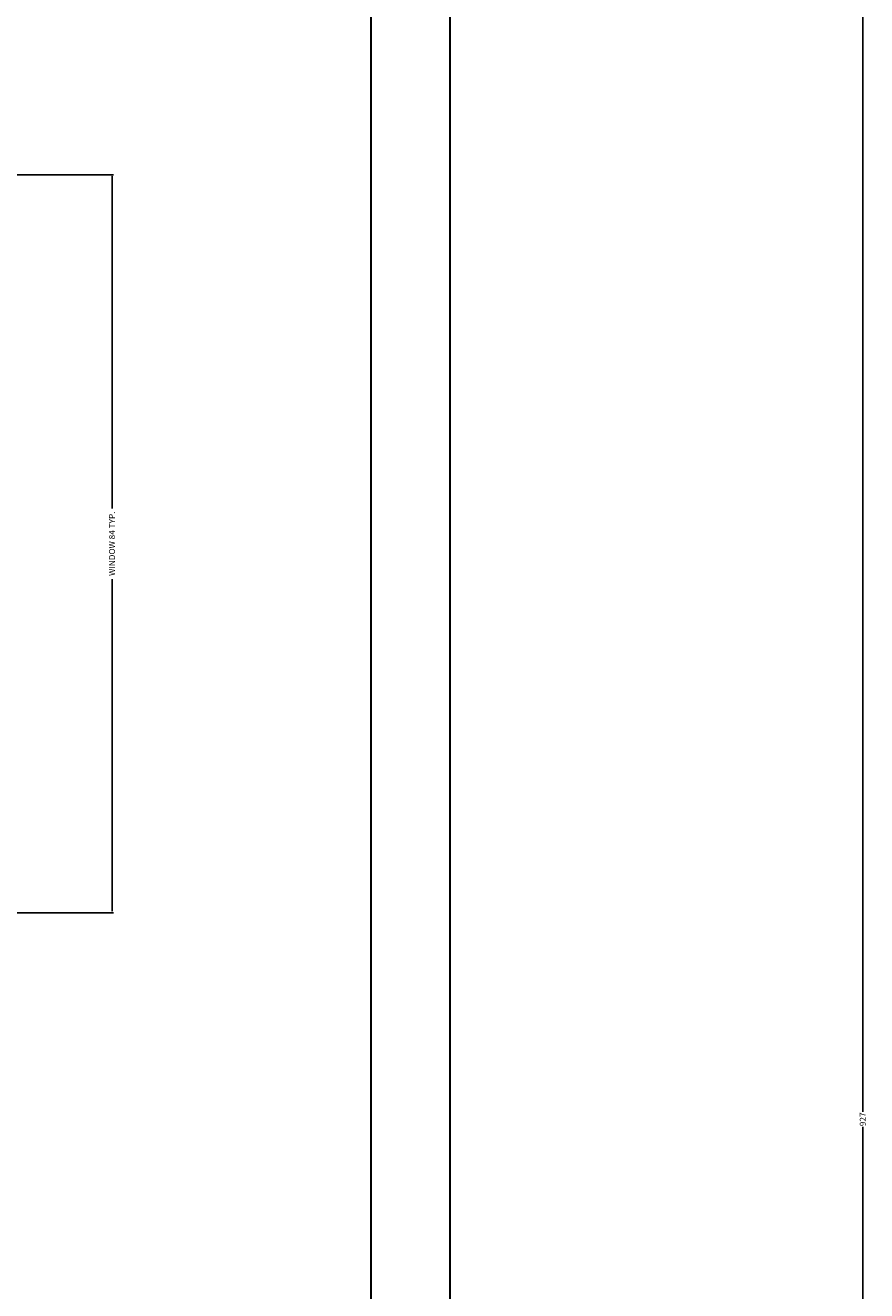
# Model space of a CAD drawing. Units: inches. Extents: x 867 to 1667, y -234 to 788.
# Tile 37 of 42: x 1572 to 1667, y 258 to 401. Entities that reach past the tile are written whole.
import ezdxf

# ---------------------------------------------------------------- set-up
doc = ezdxf.new("R2010")
doc.units = ezdxf.units.IN
doc.header["$MEASUREMENT"] = 0
doc.layers.add('A-ANNO-DIMS', color=2, linetype='Continuous', lineweight=18)
doc.layers.add('A-WALL-SITE', color=8, linetype='Continuous', lineweight=30)
doc.styles.get("Standard").update_dxf_attribs({"font": 'arial.ttf'})
doc.dimstyles.get("Standard").update_dxf_attribs({"dimtxt": 0.6875, "dimasz": 0.18, "dimexe": 0.18, "dimexo": 0.0625, "dimgap": 0.09, "dimtad": 0, "dimdec": 4, "dimzin": 0, "dimdsep": 46, "dimlunit": 4, "dimtxsty": 'Standard', "dimcen": 0.09, "dimadec": 0, "dimazin": 0, "dimtfac": 1, "dimtdec": 4, "dimtofl": 0, "dimtmove": 0, "dimatfit": 3, "dimfxl": 1, "dimtolj": 1, "dimtzin": 0, "dimarcsym": 0})

# ---------------------------------------------------------------- blocks, each defined once
blk = doc.blocks.new('*D15')
at = {"layer": 'A-ANNO-DIMS', "color": 0, "lineweight": -2, "transparency": 16777216}
for p, q in [((1568.95, 384.49), (1581.65, 384.49)), ((1581.47, 384.31), (1581.47, 346.55)), ((1581.47, 300.77), (1581.47, 338.52)), ((1568.95, 300.59), (1581.65, 300.59))]:
    blk.add_line(p, q, dxfattribs=at)
at = {"layer": 'A-ANNO-DIMS', "color": 0, "transparency": 16777216}
for points in [[(1581.44, 384.31), (1581.5, 384.31), (1581.47, 384.49)], [(1581.44, 300.77), (1581.5, 300.77), (1581.47, 300.59)]]:
    blk.add_solid(points, dxfattribs=at)
at = {"layer": 'Defpoints', "color": 0, "transparency": 16777216}
for p in [(1568.89, 384.49), (1581.47, 384.49), (1568.89, 300.59)]:
    blk.add_point(p, dxfattribs=at)
at = {"layer": 'A-ANNO-DIMS', "color": 0, "transparency": 16777216, "insert": (1581.47, 342.54), "char_height": 0.6875, "attachment_point": 5, "rotation": 90}
blk.add_mtext('\\A1;WINDOW 84 TYP.', dxfattribs=at)
blk = doc.blocks.new('*D18')
at = {"layer": 'A-ANNO-DIMS', "color": 0, "lineweight": -2, "transparency": 16777216}
for p, q in [((1619.95, 740.62), (1667.02, 740.62)), ((1666.84, 740.44), (1666.84, 277.95)), ((1666.84, -186.23), (1666.84, 276.25)), ((1619.95, -186.41), (1667.02, -186.41))]:
    blk.add_line(p, q, dxfattribs=at)
at = {"layer": 'A-ANNO-DIMS', "color": 0, "transparency": 16777216}
for points in [[(1666.81, 740.44), (1666.87, 740.44), (1666.84, 740.62)], [(1666.81, -186.23), (1666.87, -186.23), (1666.84, -186.41)]]:
    blk.add_solid(points, dxfattribs=at)
at = {"layer": 'Defpoints', "color": 0, "transparency": 16777216}
for p in [(1619.89, 740.62), (1666.84, 740.62), (1619.89, -186.41)]:
    blk.add_point(p, dxfattribs=at)
at = {"layer": 'A-ANNO-DIMS', "color": 0, "transparency": 16777216, "insert": (1666.84, 277.1), "char_height": 0.688, "attachment_point": 5, "rotation": 90}
blk.add_mtext('\\A1;927', dxfattribs=at)

msp = doc.modelspace()

# ---------------------------------------------------------------- linework, layer by layer
at = {"layer": 'A-WALL-SITE'}
for p, q in [((1610.8866, 740.617), (1610.8866, -186.4081)), ((1619.8866, 740.617), (1619.8866, -186.4081))]:
    msp.add_line(p, q, dxfattribs=at)

# ---------------------------------------------------------------- dimensions: what is measured, and where the dimension line sits
at = {"layer": 'A-ANNO-DIMS'}
dim = msp.add_linear_dim(base=(1666.8366, 740.617), p1=(1619.8866, -186.4081), p2=(1619.8866, 740.617), angle=90, dimstyle='Standard', override={"dimdec": 0, "dimlfac": 1, "dimrnd": 0, "dimzin": 0, "dimdsep": 46, "dimlunit": 2}, dxfattribs=at)
dim.commit()
dim.dimension.update_dxf_attribs({"geometry": '*D18', "text_midpoint": (1666.8366, 277.1045)})
dim = msp.add_linear_dim(base=(1581.472, 384.4878), p1=(1568.8866, 300.5856), p2=(1568.8866, 384.4878), angle=90, text='WINDOW <> TYP.', dimstyle='Standard', override={"dimdec": 0, "dimlfac": 1, "dimrnd": 0, "dimzin": 0, "dimdsep": 46, "dimlunit": 2}, dxfattribs=at)
dim.commit()
dim.dimension.update_dxf_attribs({"geometry": '*D15', "text_midpoint": (1581.472, 342.5367)})

doc.saveas('drawing.dxf')
